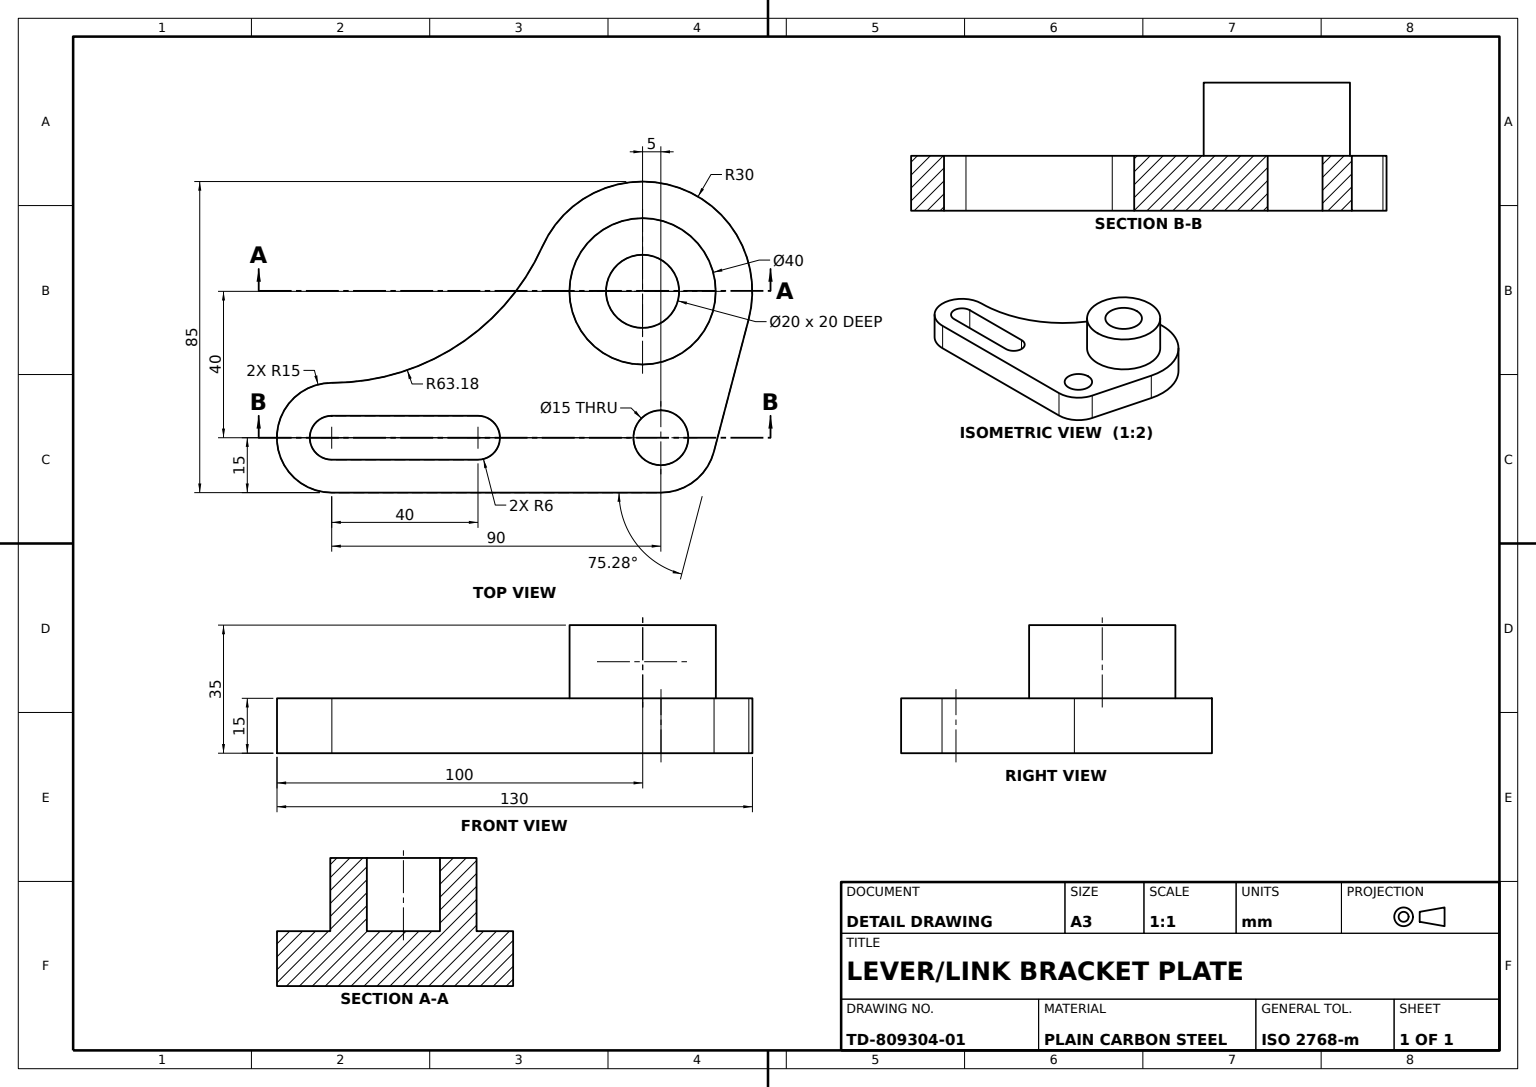
from build123d import *

# Parameters (mm, degrees)
LINK_PLATE_15MM_DEPTH        = 15
SLOT_CUT_DEPTH               = 136.462171841
THROUGH_HOLE_PROFILE_R       = 7.5
THROUGH_HOLE_CUT_DEPTH       = 15
PIVOT_BOSS_PROFILE_40_20_R   = 20
PIVOT_BOSS_PROFILE_40_20_R_2 = 10
PIVOT_BOSS_40_DEPTH          = 20


with BuildPart() as part:
    # Link Plate Profile → Link Plate 15mm (new body)
    with BuildSketch(Plane(origin=(0, 0, 0), x_dir=(1, 0, 0), z_dir=(0, 1, 0))):
        with BuildLine():
            Line((114.015316087, 32.376914511), (104.507658043, -3.811542745))
            ThreePointArc((104.507658043, -3.811542745), (99.16042736, -11.877986807), (90, -15))
            Line((90, -15), (0, -15))
            ThreePointArc((0, -15), (-15, 0), (0, 15))
            ThreePointArc((0, 15), (34.323603484, 25.136249162), (57.634146341, 52.292682927))
            ThreePointArc((57.634146341, 52.292682927), (94.991978757, 68.287105906), (114.015316087, 32.376914511))
        make_face()
    extrude(amount=LINK_PLATE_15MM_DEPTH)

    # Slot Profile → Slot Cut (cut, through all)
    with BuildSketch(Plane(origin=(0, 15, 0), x_dir=(1, 0, 0), z_dir=(0, 1, 0))):
        with BuildLine():
            Line((0, 6), (40, 6))
            ThreePointArc((40, 6), (46, 0), (40, -6))
            Line((40, -6), (0, -6))
            ThreePointArc((0, -6), (-6, 0), (0, 6))
        make_face()
    extrude(amount=-SLOT_CUT_DEPTH, mode=Mode.SUBTRACT)

    # Through Hole Profile → Through Hole Cut (cut)
    with BuildSketch(Plane(origin=(0, 15, 0), x_dir=(1, 0, 0), z_dir=(0, 1, 0))):
        with Locations(Location((90, 0, 0), (0, 0, 270))):
            Circle(THROUGH_HOLE_PROFILE_R)
    extrude(amount=-THROUGH_HOLE_CUT_DEPTH, mode=Mode.SUBTRACT)

    # Pivot Boss Profile Ø40-Ø20 → Pivot Boss Ø40 (add)
    with BuildSketch(Plane(origin=(0, 15, 0), x_dir=(1, 0, 0), z_dir=(0, 1, 0))):
        with Locations(Location((85, 40, 0), (0, 0, 270))):
            Circle(PIVOT_BOSS_PROFILE_40_20_R)
        with Locations(Location((85, 40, 0), (0, 0, 270))):
            Circle(PIVOT_BOSS_PROFILE_40_20_R_2, mode=Mode.SUBTRACT)
    extrude(amount=PIVOT_BOSS_40_DEPTH)


solid = part.part
